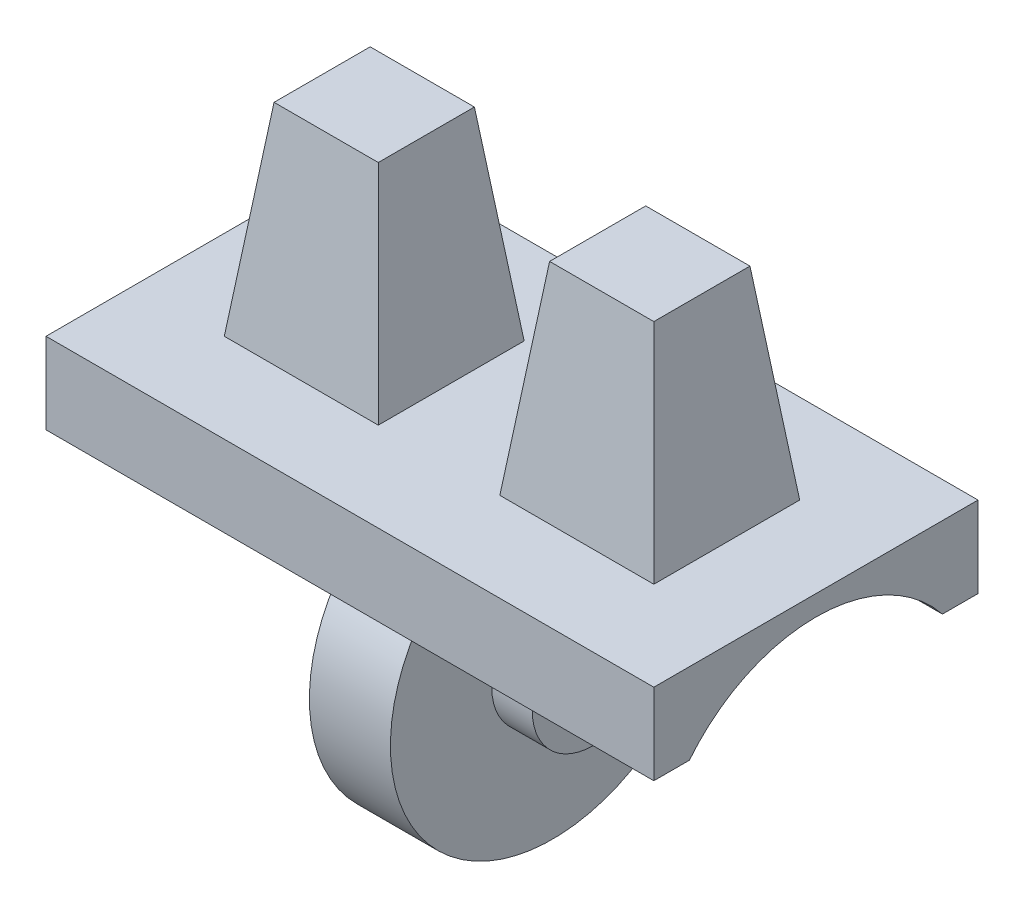
from build123d import *

# Parameters (mm, degrees)
BASE_PLATE_SKETCH_W                    = 15
BASE_PLATE_SKETCH_H                    = 8
BASE_PLATE_15X8X2_DEPTH                = 2
HIP_BLOCKS_SKETCH_W                    = 3.8
HIP_BLOCKS_SKETCH_H                    = 3.6
HIP_BLOCKS_DRAFTED_5MM_DEPTH           = 5
HIP_BLOCKS_DRAFTED_5MM_DRAFT           = 7
HIP_BLOCKS_DRAFTED_5MM_PROFILE_2_DEPTH = 5
HIP_BLOCKS_DRAFTED_5MM_PROFILE_2_DRAFT = 7
UNDERSIDE_RELIEF_SKETCH_R              = 4
UNDERSIDE_RELIEF_CUT_DEPTH             = 19.384776311
HIP_DISC_SKETCH_R                      = 4
HIP_DISC_8_DEPTH                       = 1
AXLE_PIN_A_SKETCH_R                    = 1.5
AXLE_PIN_A_3_DEPTH                     = 1
AXLE_PIN_B_SKETCH_R                    = 1.5
AXLE_PIN_B_3_DEPTH                     = 1


with BuildPart() as part:
    # Base Plate Sketch → Base Plate 15x8x2 (new body)
    with BuildSketch(Plane(origin=(0, 0, 0), x_dir=(1, 0, 0), z_dir=(0, 1, 0))):
        with Locations((7.5, 4)):
            Rectangle(BASE_PLATE_SKETCH_W, BASE_PLATE_SKETCH_H)
    extrude(amount=BASE_PLATE_15X8X2_DEPTH)


with BuildPart() as hip_blocks_drafted_5mm_tool:
    # Hip Blocks Sketch → Hip Blocks Drafted 5mm (with draft: the straight prism first)
    with BuildSketch(Plane(origin=(0, 2, 0), x_dir=(1, 0, 0), z_dir=(0, 1, 0))):
        with Locations((4.1, 4)):
            Rectangle(HIP_BLOCKS_SKETCH_W, HIP_BLOCKS_SKETCH_H)
    extrude(amount=HIP_BLOCKS_DRAFTED_5MM_DEPTH)
    # Hip Blocks Drafted 5mm: the draft: its side faces are tilted about the plane it starts from
    hip_blocks_drafted_5mm_sides = [hip_blocks_drafted_5mm_tool.faces().sort_by_distance(p)[0] for p in [
        (2.2, 4.5, -4),
        (4.1, 4.5, -2.2),
        (6, 4.5, -4),
        (4.1, 4.5, -5.8),
    ]]
    draft(hip_blocks_drafted_5mm_sides, Plane(origin=(0, 2, 0), x_dir=(1, 0, 0), z_dir=(0, 1, 0)), HIP_BLOCKS_DRAFTED_5MM_DRAFT)


with BuildPart() as part_1:
    add(part.part)

    # Hip Blocks Drafted 5mm: add hip_blocks_drafted_5mm_tool
    add(hip_blocks_drafted_5mm_tool.part)


with BuildPart() as hip_blocks_drafted_5mm_profile_2_tool:
    # Hip Blocks Sketch → Hip Blocks Drafted 5mm profile 2 (with draft: the straight prism first)
    with BuildSketch(Plane(origin=(0, 2, 0), x_dir=(1, 0, 0), z_dir=(0, 1, 0))):
        with Locations((10.9, 4)):
            Rectangle(HIP_BLOCKS_SKETCH_W, HIP_BLOCKS_SKETCH_H)
    extrude(amount=HIP_BLOCKS_DRAFTED_5MM_PROFILE_2_DEPTH)
    # Hip Blocks Drafted 5mm profile 2: the draft: its side faces are tilted about the plane it starts from
    hip_blocks_drafted_5mm_profile_2_sides = [hip_blocks_drafted_5mm_profile_2_tool.faces().sort_by_distance(p)[0] for p in [
        (10.9, 4.5, -5.8),
        (9, 4.5, -4),
        (10.9, 4.5, -2.2),
        (12.8, 4.5, -4),
    ]]
    draft(hip_blocks_drafted_5mm_profile_2_sides, Plane(origin=(0, 2, 0), x_dir=(1, 0, 0), z_dir=(0, 1, 0)), HIP_BLOCKS_DRAFTED_5MM_PROFILE_2_DRAFT)


with BuildPart() as part_2:
    add(part_1.part)

    # Hip Blocks Drafted 5mm profile 2: add hip_blocks_drafted_5mm_profile_2_tool
    add(hip_blocks_drafted_5mm_profile_2_tool.part)

    # Underside Relief Sketch → Underside Relief Cut (cut, through all)
    with BuildSketch(Plane(origin=(15, 0, 0), x_dir=(0, 0, -1), z_dir=(1, 0, 0))):
        with Locations((4, -2.5)):
            Circle(UNDERSIDE_RELIEF_SKETCH_R)
    extrude(amount=-UNDERSIDE_RELIEF_CUT_DEPTH, mode=Mode.SUBTRACT)

    # Hip Disc Sketch → Hip Disc Ø8 (add, symmetric)
    with BuildSketch(Plane.ZY.offset(-7.5)):
        with Locations((-4, -2.5)):
            Circle(HIP_DISC_SKETCH_R)
    extrude(amount=HIP_DISC_8_DEPTH, both=True)

    # Axle Pin A Sketch → Axle Pin A Ø3 (add, symmetric)
    with BuildSketch(Plane(origin=(8.5, 0, 0), x_dir=(0, 0, -1), z_dir=(1, 0, 0))):
        with Locations(Location((4, -2.5, 0), (0, 0, 180))):
            Circle(AXLE_PIN_A_SKETCH_R)
    extrude(amount=AXLE_PIN_A_3_DEPTH, both=True)

    # Axle Pin B Sketch → Axle Pin B Ø3 (add, symmetric)
    with BuildSketch(Plane.ZY.offset(-6.5)):
        with Locations((-4, -2.5)):
            Circle(AXLE_PIN_B_SKETCH_R)
    extrude(amount=AXLE_PIN_B_3_DEPTH, both=True)


solid = part_2.part
